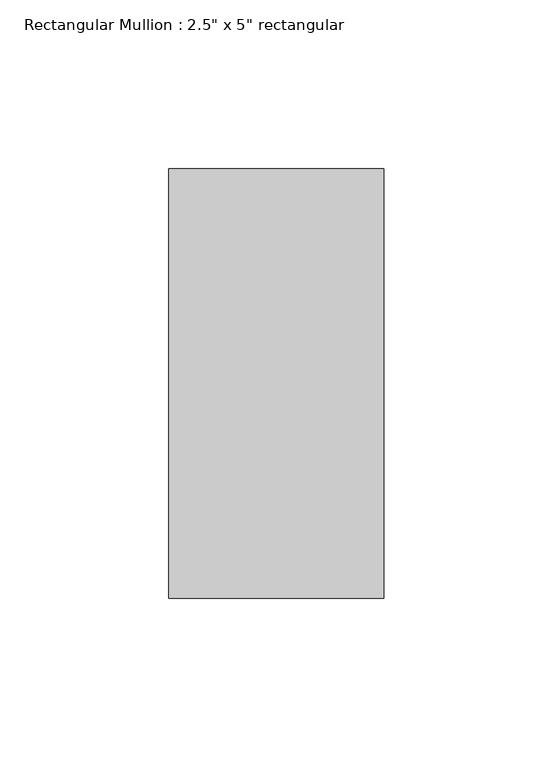
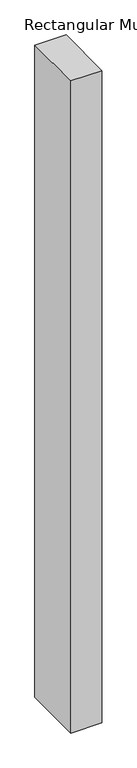
"""IFC4 building model written with IfcOpenShell, lengths in millimetres: member geometry."""

from ifc_helpers import new_model, si_unit, frame, origin, place, context, project, spatial, polyline, outline, extrude, source, transform, mapped, element, save


def member_36d9a658(model_context):
    return source(origin(), model_context, "Body", "SweptSolid", [
        extrude(outline(polyline([(0.0, 63.5), (0.0, -63.5), (-63.5, -63.5), (-63.5, 63.5), (0.0, 63.5)])), frame((0.0, 0.0, -1406.4174829), z_axis=(0.0, 0.0, 1.0), x_axis=(1.0, 0.0, 0.0)), (0.0, 0.0, 1.0), 1406.4174829),
    ])


if __name__ == "__main__":
    model = new_model("IFC4")
    model_context = context("Model", 3, world=origin())
    ifc_project = project(units=[si_unit("LENGTHUNIT", "METRE", prefix="MILLI")], contexts=[model_context])
    site = spatial("IfcSite", under=ifc_project)
    building = spatial("IfcBuilding", under=site)
    placement = place(None, origin())
    member_shape = member_36d9a658(model_context)
    element("IfcMember", 1, ObjectType="Rectangular Mullion : 2.5\" x 5\" rectangular", at=placement, inside=building, context=model_context, shape_type="MappedRepresentation", body=[
        mapped(member_shape, transform((0.0, 0.0, 0.0), x_axis=(1.0, 0.0, 0.0), y_axis=(0.0, 1.0, 0.0), z_axis=(0.0, 0.0, 1.0))),
    ])
    save(model, "model.ifc")

# Revit data of these elements
# Type "Rectangular Mullion : 2.5\" x 5\" rectangular"
#   built-in parameter 1007304 = 0.416667 (stored number, unit not read)
#   built-in parameter 1007301 = 0.104167 (stored number, unit not read)
#   built-in parameter 1007300 = 0.104167 (stored number, unit not read)
# Element 1 (IfcMember, "Rectangular Mullion : 2.5\" x 5\" rectangular")
#   Materials on its faces: "Aluminum"
# Materials
#   "Aluminum": class "Metal", colour RGB 247 247 247, transparency 0, Description = "Aluminum 6061", Cost = 0
